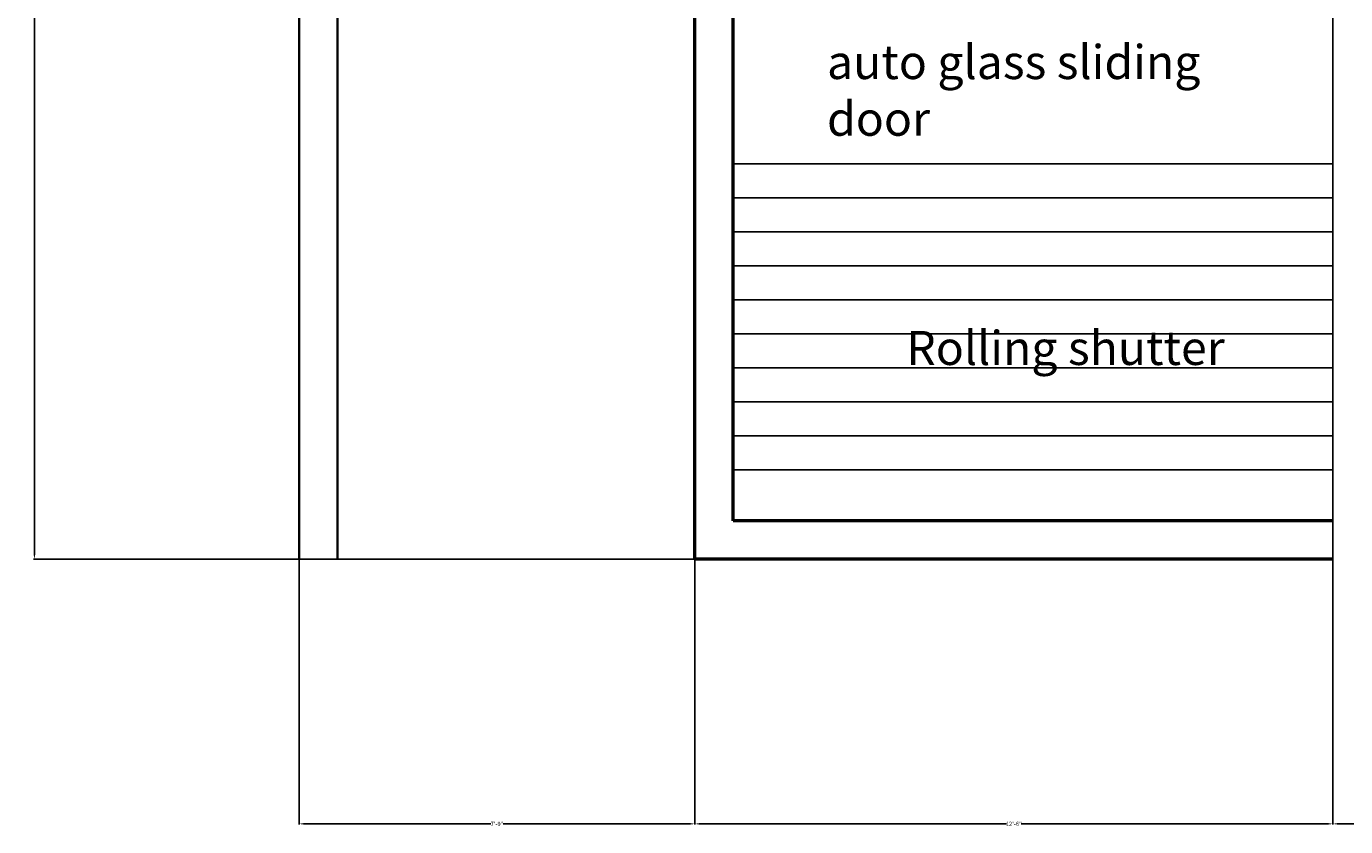
# Model space of a CAD drawing. Units: inches. Extents: x -364 to 705, y -52 to 1250.
# Tile 2 of 34: x -129 to 182, y -52 to 136. Entities that reach past the tile are written whole.
import ezdxf

# ---------------------------------------------------------------- set-up
doc = ezdxf.new("R2010")
doc.units = ezdxf.units.IN
doc.header["$MEASUREMENT"] = 0
for name, color, linetype, lineweight in [('A-ANNO-DIMS', 4, 'Continuous', 18), ('A-ANNO-TEXT', 3, 'Continuous', 18), ('A-DOOR', 1, 'Continuous', 25), ('A-FLOR-RAMP', 7, 'Continuous', 25), ('A-WALL', 41, 'Continuous', 50), ('C-WALL', 41, 'Continuous', 35)]:
    doc.layers.add(name, color=color, linetype=linetype, lineweight=lineweight)
doc.styles.get("Standard").update_dxf_attribs({"font": 'arial.ttf'})
doc.dimstyles.get("Standard").update_dxf_attribs({"dimtxt": 1, "dimasz": 1, "dimexe": 0.18, "dimexo": 0.0625, "dimgap": 0.09, "dimtad": 0, "dimtih": 1, "dimtoh": 1, "dimdec": 0, "dimzin": 0, "dimdsep": 46, "dimlunit": 3, "dimtxsty": 'Standard', "dimcen": 0.09, "dimadec": 0, "dimazin": 0, "dimtfac": 1, "dimtdec": 0, "dimtofl": 0, "dimtmove": 0, "dimatfit": 3, "dimfxl": 1, "dimtolj": 1, "dimtzin": 0, "dimarcsym": 0})

# ---------------------------------------------------------------- blocks, each defined once
blk = doc.blocks.new('*D76')
at = {"layer": 'A-ANNO-DIMS', "color": 0, "lineweight": -2, "transparency": 16777216}
for p, q in [((28.52, 986.11), (-126.85, 986.11)), ((-126.67, 985.11), (-126.67, 499.22)), ((-126.67, 12.11), (-126.67, 498.01)), ((28.52, 11.11), (-126.85, 11.11))]:
    blk.add_line(p, q, dxfattribs=at)
at = {"layer": 'A-ANNO-DIMS', "color": 0, "transparency": 16777216}
for points in [[(-126.84, 985.11), (-126.5, 985.11), (-126.67, 986.11)], [(-126.84, 12.11), (-126.5, 12.11), (-126.67, 11.11)]]:
    blk.add_solid(points, dxfattribs=at)
at = {"layer": 'Defpoints', "color": 0, "transparency": 16777216}
for p in [(-126.67, 986.11), (28.58, 986.11), (28.58, 11.11)]:
    blk.add_point(p, dxfattribs=at)
at = {"layer": 'A-ANNO-DIMS', "color": 0, "transparency": 16777216, "insert": (-126.67, 498.61), "char_height": 1, "attachment_point": 5}
blk.add_mtext('\\A1;81\'-3"', dxfattribs=at)
blk = doc.blocks.new('*D85')
at = {"layer": 'A-ANNO-DIMS', "color": 0, "lineweight": -2, "transparency": 16777216}
for p, q in [((28.58, 11.05), (28.58, -51.32)), ((178.58, 11.05), (178.58, -51.32)), ((29.58, -51.14), (101.82, -51.14)), ((177.58, -51.14), (105.34, -51.14))]:
    blk.add_line(p, q, dxfattribs=at)
at = {"layer": 'A-ANNO-DIMS', "color": 0, "transparency": 16777216}
for points in [[(29.58, -50.97), (29.58, -51.3), (28.58, -51.14)], [(177.58, -50.97), (177.58, -51.3), (178.58, -51.14)]]:
    blk.add_solid(points, dxfattribs=at)
at = {"layer": 'Defpoints', "color": 0, "transparency": 16777216}
for p in [(28.58, 11.11), (178.58, 11.11), (178.58, -51.14)]:
    blk.add_point(p, dxfattribs=at)
at = {"layer": 'A-ANNO-DIMS', "color": 0, "transparency": 16777216, "insert": (103.58, -51.14), "char_height": 1, "attachment_point": 5}
blk.add_mtext('\\A1;12\'-6"', dxfattribs=at)
blk = doc.blocks.new('*D86')
at = {"layer": 'A-ANNO-DIMS', "color": 0, "lineweight": -2, "transparency": 16777216}
for p, q in [((178.58, 11.05), (178.58, -51.32)), ((226.58, 11.05), (226.58, -51.32)), ((179.58, -51.14), (201.14, -51.14)), ((225.58, -51.14), (204.02, -51.14))]:
    blk.add_line(p, q, dxfattribs=at)
at = {"layer": 'A-ANNO-DIMS', "color": 0, "transparency": 16777216}
for points in [[(179.58, -50.97), (179.58, -51.3), (178.58, -51.14)], [(225.58, -50.97), (225.58, -51.3), (226.58, -51.14)]]:
    blk.add_solid(points, dxfattribs=at)
at = {"layer": 'Defpoints', "color": 0, "transparency": 16777216}
for p in [(178.58, 11.11), (226.58, 11.11), (226.58, -51.14)]:
    blk.add_point(p, dxfattribs=at)
at = {"layer": 'A-ANNO-DIMS', "color": 0, "transparency": 16777216, "insert": (202.58, -51.14), "char_height": 1, "attachment_point": 5}
blk.add_mtext('\\A1;4\'-0"', dxfattribs=at)
blk = doc.blocks.new('*D90')
at = {"layer": 'A-ANNO-DIMS', "color": 0, "lineweight": -2, "transparency": 16777216}
for p, q in [((-64.42, 11.05), (-64.42, -51.32)), ((28.58, 11.05), (28.58, -51.32)), ((-63.42, -51.14), (-19.33, -51.14)), ((27.58, -51.14), (-16.5, -51.14))]:
    blk.add_line(p, q, dxfattribs=at)
at = {"layer": 'A-ANNO-DIMS', "color": 0, "transparency": 16777216}
for points in [[(-63.42, -50.97), (-63.42, -51.3), (-64.42, -51.14)], [(27.58, -50.97), (27.58, -51.3), (28.58, -51.14)]]:
    blk.add_solid(points, dxfattribs=at)
at = {"layer": 'Defpoints', "color": 0, "transparency": 16777216}
for p in [(-64.42, 11.11), (28.58, 11.11), (28.58, -51.14)]:
    blk.add_point(p, dxfattribs=at)
at = {"layer": 'A-ANNO-DIMS', "color": 0, "transparency": 16777216, "insert": (-17.92, -51.14), "char_height": 1, "attachment_point": 5}
blk.add_mtext('\\A1;7\'-9"', dxfattribs=at)

msp = doc.modelspace()

# ---------------------------------------------------------------- linework, layer by layer
at = {"layer": 'A-DOOR'}
for p, q in [((178.58, 104.11), (37.58, 104.11)), ((178.58, 96.11), (37.58, 96.11)), ((178.58, 88.11), (37.58, 88.11)), ((178.58, 80.11), (37.58, 80.11)), ((178.58, 72.11), (37.58, 72.11)), ((178.58, 64.11), (37.58, 64.11)), ((178.58, 56.11), (37.58, 56.11)), ((178.58, 48.11), (37.58, 48.11)), ((178.58, 40.11), (37.58, 40.11)), ((178.58, 32.11), (37.58, 32.11))]:
    msp.add_line(p, q, dxfattribs=at)
at = {"layer": 'A-FLOR-RAMP'}
msp.add_line((178.58, 11.11), (178.58, 149.11), dxfattribs=at)
at = {"layer": 'A-WALL'}
for p, q in [((28.58, 11.11), (28.58, 986.11)), ((37.58, 20.11), (37.58, 140.11)), ((178.58, 20.11), (37.58, 20.11)), ((178.58, 11.11), (28.58, 11.11))]:
    msp.add_line(p, q, dxfattribs=at)
at = {"layer": 'C-WALL'}
for p, q in [((-64.42, 11.11), (-64.42, 1079.11)), ((-55.42, 11.11), (-55.42, 1070.11))]:
    msp.add_line(p, q, dxfattribs=at)

# ---------------------------------------------------------------- texts
at = {"layer": 'A-ANNO-TEXT', "char_height": 8, "attachment_point": 1}
for s, width, insert in [('auto glass sliding door', 104.3269, (59.66, 132.02)), ('Rolling shutter', 76.2228, (78.3, 64.78))]:
    msp.add_mtext_dynamic_manual_height_columns(s, width=width, gutter_width=1, heights=[0], dxfattribs=dict(at, insert=insert))

# ---------------------------------------------------------------- dimensions: what is measured, and where the dimension line sits
at = {"layer": 'A-ANNO-DIMS'}
dim = msp.add_linear_dim(base=(-126.67, 986.11), p1=(28.58, 11.11), p2=(28.58, 986.11), angle=90, dimstyle='Standard', override={"dimdec": 1, "dimlfac": 1, "dimrnd": 0, "dimzin": 1, "dimdsep": 46, "dimlunit": 4, "dimfrac": 2}, dxfattribs=at)
dim.commit()
dim.dimension.update_dxf_attribs({"geometry": '*D76', "text_midpoint": (-126.67, 498.61)})
for base, p1, p2, picture, middle in [((28.58, -51.14), (-64.42, 11.11), (28.58, 11.11), '*D90', (-17.92, -51.14)), ((178.58, -51.14), (28.58, 11.11), (178.58, 11.11), '*D85', (103.58, -51.14)), ((226.58, -51.14), (178.58, 11.11), (226.58, 11.11), '*D86', (202.58, -51.14))]:
    dim = msp.add_linear_dim(base=base, p1=p1, p2=p2, dimstyle='Standard', override={"dimdec": 1, "dimlfac": 1, "dimrnd": 0, "dimzin": 1, "dimdsep": 46, "dimlunit": 4, "dimfrac": 2}, dxfattribs=at)
    dim.commit()
    dim.dimension.update_dxf_attribs({"geometry": picture, "text_midpoint": middle})

doc.saveas('drawing.dxf')
